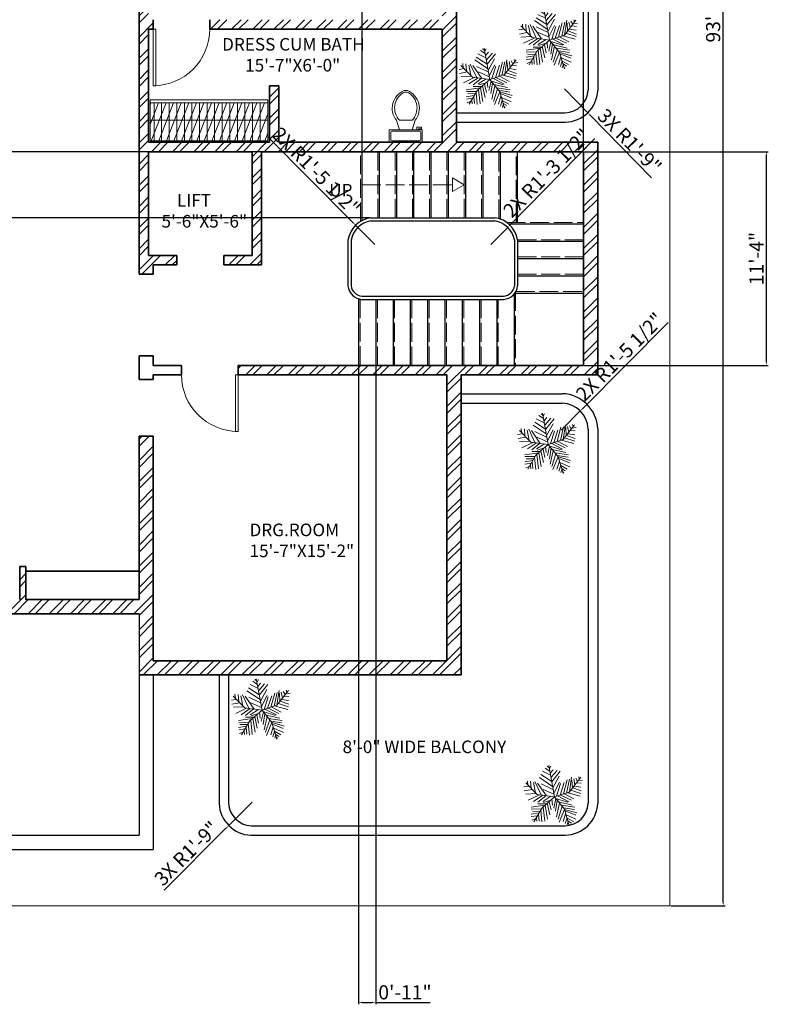
# Model space of a CAD drawing. Units: inches. Extents: x 155 to 1269, y 1260 to 2528.
# Tile 4 of 6: x 792 to 1269, y 1277 to 1903. Entities that reach past the tile are written whole.
import ezdxf

# ---------------------------------------------------------------- set-up
doc = ezdxf.new("R2010")
doc.units = ezdxf.units.IN
doc.linetypes.add('ACAD_ISO02W100', pattern=[15, 12, -3])
for name, color, linetype, lineweight in [('A-ANNO-DIMS', 2, 'Continuous', 18), ('A-ANNO-SYMB', 7, 'Continuous', 18), ('A-ANNO-TEXT', 7, 'Continuous', 25), ('A-AREA-IDEN', 7, 'Continuous', 18), ('A-DOOR', 3, 'Continuous', 18), ('A-FLOR-CASE', 9, 'Continuous', 18), ('A-FLOR-CASE-PATT', 252, 'Continuous', 13), ('A-FLOR-EDGE', 7, 'Continuous', 25), ('A-FLOR-FIXT', 9, 'Continuous', 18), ('A-FLOR-STRS', 7, 'Continuous', 25), ('A-FLOR-STRS-HIDN', 8, 'ACAD_ISO02W100', 13), ('A-FLOR-STRS-PATH', 7, 'ACAD_ISO02W100', 18), ('A-WALL', 7, 'Continuous', 35), ('A-WALL-PATT', 252, 'Continuous', 13), ('C-PROP', 8, 'Continuous', 18), ('L-PLNT', 94, 'Continuous', 13)]:
    doc.layers.add(name, color=color, linetype=linetype, lineweight=lineweight)
doc.styles.get("Standard").update_dxf_attribs({"font": 'arial.ttf'})
doc.dimstyles.new('ISO-25', dxfattribs={"dimtxt": 9, "dimasz": 2.5, "dimexe": 1.25, "dimexo": 0.625, "dimtad": 1, "dimlunit": 3, "dimtxsty": 'Standard', "dimcen": 2.5, "dimadec": 0, "dimazin": 0, "dimtfac": 1, "dimtmove": 0, "dimatfit": 3, "dimfxl": 1, "dimarcsym": 0})

# ---------------------------------------------------------------- blocks, each defined once
blk = doc.blocks.new('*U4')
for p, q in [((-40, 0), (-40, 6)), ((0, 0), (0, 6))]:
    blk.add_line(p, q)
blk.add_lwpolyline([(0, 0), (0, -40), (-1.75, -40), (-1.75, 0)], close=True)
blk.add_arc((0, 0), 40, 180, 270)
blk = doc.blocks.new('*U8')
for p, q in [((9.5, -6), (9.5, -2)), ((-10, -8.5), (-8, -8.5)), ((-10, -9.5), (-10, -8.5)), ((-7, -9.5), (-10, -9.5)), ((-8, -8.5), (-8, -8)), ((-7, -8), (-7, -9.5)), ((-4, -8), (-6, -14)), ((4, -8), (6, -14)), ((4, -14), (-4, -14))]:
    blk.add_line(p, q)
blk.add_lwpolyline([(10.5, -8), (10.5, 0), (-10.5, 0), (-10.5, -8)], close=True)
for points in [[(-9.5, -2), (-9.5, -6)], [(8.5, -1), (-8.5, -1)], [(-8.5, -7), (8.5, -7)]]:
    blk.add_lwpolyline(points)
for centre, radius, start, end in [((-8.62, -1.88), 0.884, 81.8699, 188.1301), ((-8.62, -6.12), 0.884, 171.8699, 278.1301), ((8.62, -1.88), 0.884, 351.8699, 98.1301), ((8.62, -6.12), 0.884, 261.8699, 8.1301), ((3.52, -21.58), 12.17, 141.46911, 247.97143), ((4.2, -21.82), 11.33, 136.36773, 238.94682), ((-3.52, -21.58), 12.17, 292.02843, 38.53071), ((-4.2, -21.82), 11.33, 301.05301, 43.63209), ((0, -27.88), 4, 245.73182, 294.26817), ((0, -29), 4, 254.86053, 285.13947)]:
    blk.add_arc(centre, radius, start, end)
blk = doc.blocks.new('*U9')
for p, q in [((0, 0), (0, 6)), ((40, 0), (40, 6))]:
    blk.add_line(p, q)
blk.add_lwpolyline([(0, 0), (0, -40), (1.75, -40), (1.75, 0)], close=True)
blk.add_arc((0, 0), 40, 270, 0)
blk = doc.blocks.new('*U11')
for p, q in [((-10.186, 53.64), (-13.084, 55.962)), ((0, 0), (-10.5, 57)), ((-9.099, 51.782), (-6.563, 55.962)), ((-5.114, 28.097), (-24.676, 40.636)), ((-7.288, 39.707), (-21.778, 46.673)), ((-8.737, 47.138), (-17.069, 52.711)), ((-7.65, 43.423), (-2.578, 49.46)), ((-5.839, 35.992), (4.667, 48.067)), ((-5.114, 27.632), (10.463, 46.673)), ((-2.941, 16.486), (8.652, 37.85)), ((27, 9), (48, 36)), ((27.127, 9.056), (31.112, 35.992)), ((44.153, 36.456), (45.239, 32.741)), ((-47.498, 19.737), (-55.83, 18.344)), ((-31.5, 4.5), (-52.5, 25.5)), ((-48.585, 21.131), (-49.309, 29.026)), ((-43.513, 28.561), (-42.427, 15.558)), ((-38.442, 26.239), (-34.819, 7.663)), ((-35.544, 28.097), (-24.314, 3.947)), ((-14.533, 2.09), (-30.834, 25.31)), ((-3.665, 19.273), (-27.574, 35.527)), ((-24.314, 23.917), (-2.941, 13.7)), ((-1.129, 6.734), (9.014, 26.704)), ((3.942, 1.625), (11.187, 24.381)), ((10.101, 3.483), (17.708, 26.239)), ((16.259, 5.805), (23.142, 31.348)), ((22.055, 7.198), (27.489, 32.277)), ((31.836, 30.883), (32.561, 16.486)), ((35.096, 32.741), (37.27, 22.524)), ((36.183, 19.737), (48.137, 17.88)), ((38.719, 34.134), (41.979, 28.561)), ((40.53, 25.775), (48.862, 24.846)), ((43.791, 29.954), (51.036, 30.883)), ((-40.615, 13.7), (-55.105, 10.913)), ((-33.37, 6.269), (-52.207, 5.34)), ((-28.299, 3.483), (-47.86, -5.805)), ((-21.416, 3.018), (-38.079, -8.128)), ((0, 0), (-31.5, 4.5)), ((-15.982, 2.09), (-30.11, -9.521)), ((0, 0), (-22.5, -19.5)), ((-6.563, 1.161), (-21.416, -8.128)), ((-20.691, 13.7), (-1.129, 4.876)), ((0, 0), (27, 9)), ((0, 0), (18, -22.5)), ((6.478, 1.625), (26.04, -8.592)), ((11.187, 3.483), (30.749, -5.805)), ((18.07, 5.805), (35.096, -3.483)), ((24.229, 7.663), (46.688, 1.625)), ((29.662, 12.307), (48.137, 6.269)), ((33.285, 16.486), (48.862, 10.913)), ((-17.431, -15.094), (-42.789, -18.809)), ((-15.257, -12.772), (-30.11, -12.772)), ((-6.563, -5.805), (-19.967, -9.985)), ((-17.069, -15.094), (-12.721, -40.172)), ((-13.446, -11.378), (-8.737, -32.741)), ((-9.461, -8.592), (-6.201, -23.453)), ((-4.752, -3.483), (-3.665, -14.629)), ((2.493, -3.019), (-1.491, -20.202)), ((1.769, -2.555), (24.229, -9.521)), ((5.029, -6.27), (2.131, -25.775)), ((9.014, -11.378), (3.58, -35.992)), ((14.085, -16.951), (6.478, -40.172)), ((7.565, -9.056), (32.198, -14.629)), ((12.274, -15.094), (36.907, -18.809)), ((-28.299, -29.026), (-42.789, -31.348)), ((-24.314, -21.596), (-42.427, -22.06)), ((-30.834, -34.135), (-42.427, -35.528)), ((-26.849, -26.24), (-40.253, -25.775)), ((-22.5, -19.5), (-37.5, -45)), ((-29.023, -30.884), (-27.936, -43.887)), ((-25.038, -23.918), (-22.865, -45.281)), ((-20.691, -18.345), (-17.793, -44.352)), ((18.07, -22.524), (8.289, -45.745)), ((20.244, -30.419), (15.897, -44.816)), ((16.259, -19.738), (36.183, -22.989)), ((18, -22.5), (27, -52.5)), ((18.433, -22.524), (40.53, -29.026)), ((19.157, -25.311), (38.719, -33.206)), ((21.331, -32.741), (39.081, -40.636)), ((-34.457, -39.708), (-40.978, -42.494)), ((-32.646, -36.921), (-31.921, -44.352)), ((22.78, -37.85), (19.519, -48.532)), ((22.78, -38.314), (34.372, -44.816)), ((24.591, -45.745), (23.142, -50.854)), ((24.591, -43.423), (30.749, -47.603)), ((26.764, -49.925), (28.213, -50.854))]:
    blk.add_line(p, q)
blk = doc.blocks.new('*D13')
at = {"layer": 'A-ANNO-DIMS', "color": 0, "lineweight": -2, "transparency": 16777216}
for p, q in [((1207.02, 2455.18), (1241.52, 2455.18)), ((1240.27, 1341.68), (1240.27, 2452.68)), ((1207.02, 1339.18), (1241.52, 1339.18))]:
    blk.add_line(p, q, dxfattribs=at)
at = {"layer": 'A-ANNO-DIMS', "color": 0, "transparency": 16777216}
for points in [[(1239.85, 2452.68), (1240.68, 2452.68), (1240.27, 2455.18)], [(1239.85, 1341.68), (1240.68, 1341.68), (1240.27, 1339.18)]]:
    blk.add_solid(points, dxfattribs=at)
at = {"layer": 'Defpoints', "color": 0, "transparency": 16777216}
for p in [(1206.4, 2455.18), (1240.27, 2455.18), (1206.4, 1339.18)]:
    blk.add_point(p, dxfattribs=at)
at = {"layer": 'A-ANNO-DIMS', "color": 0, "transparency": 16777216, "insert": (1235.04, 1897.18), "char_height": 9, "attachment_point": 5, "rotation": 90}
blk.add_mtext("93'", dxfattribs=at)
blk = doc.blocks.new('*D45')
at = {"layer": 'A-ANNO-DIMS', "color": 0, "lineweight": -2, "transparency": 16777216}
for p, q in [((1010.4, 1819.81), (1010.4, 2517.78)), ((1012.9, 2516.53), (1148.9, 2516.53)), ((1151.4, 1819.81), (1151.4, 2517.78))]:
    blk.add_line(p, q, dxfattribs=at)
at = {"layer": 'A-ANNO-DIMS', "color": 0, "transparency": 16777216}
for points in [[(1012.9, 2516.95), (1012.9, 2516.11), (1010.4, 2516.53)], [(1148.9, 2516.95), (1148.9, 2516.11), (1151.4, 2516.53)]]:
    blk.add_solid(points, dxfattribs=at)
at = {"layer": 'Defpoints', "color": 0, "transparency": 16777216}
for p in [(1151.4, 2516.53), (1010.4, 1819.18), (1151.4, 1819.18)]:
    blk.add_point(p, dxfattribs=at)
at = {"layer": 'A-ANNO-DIMS', "color": 0, "transparency": 16777216, "insert": (1080.9, 2521.75), "char_height": 9, "attachment_point": 5}
blk.add_mtext('11\'-9"', dxfattribs=at)
blk = doc.blocks.new('*D46')
at = {"layer": 'A-ANNO-DIMS', "color": 0, "lineweight": -2, "transparency": 16777216}
for p, q in [((1009.77, 1819.18), (164.8, 1819.18)), ((166.05, 1779.68), (166.05, 1816.68)), ((1015.06, 1777.18), (164.8, 1777.18))]:
    blk.add_line(p, q, dxfattribs=at)
at = {"layer": 'A-ANNO-DIMS', "color": 0, "transparency": 16777216}
for points in [[(165.63, 1816.68), (166.46, 1816.68), (166.05, 1819.18)], [(165.63, 1779.68), (166.46, 1779.68), (166.05, 1777.18)]]:
    blk.add_solid(points, dxfattribs=at)
at = {"layer": 'Defpoints', "color": 0, "transparency": 16777216}
for p in [(166.05, 1819.18), (1010.4, 1819.18), (1015.68, 1777.18)]:
    blk.add_point(p, dxfattribs=at)
at = {"layer": 'A-ANNO-DIMS', "color": 0, "transparency": 16777216, "insert": (160.82, 1798.18), "char_height": 9, "attachment_point": 5, "rotation": 90}
blk.add_mtext('3\'-6"', dxfattribs=at)
blk = doc.blocks.new('*D47')
at = {"layer": 'A-ANNO-DIMS', "color": 0, "lineweight": -2, "transparency": 16777216}
for p, q in [((1152.02, 1819.18), (1269, 1819.18)), ((1267.75, 1685.68), (1267.75, 1816.68)), ((1152.02, 1683.18), (1269, 1683.18))]:
    blk.add_line(p, q, dxfattribs=at)
at = {"layer": 'A-ANNO-DIMS', "color": 0, "transparency": 16777216}
for points in [[(1267.33, 1816.68), (1268.16, 1816.68), (1267.75, 1819.18)], [(1267.33, 1685.68), (1268.16, 1685.68), (1267.75, 1683.18)]]:
    blk.add_solid(points, dxfattribs=at)
at = {"layer": 'Defpoints', "color": 0, "transparency": 16777216}
for p in [(1151.4, 1819.18), (1267.75, 1819.18), (1151.4, 1683.18)]:
    blk.add_point(p, dxfattribs=at)
at = {"layer": 'A-ANNO-DIMS', "color": 0, "transparency": 16777216, "insert": (1262.6, 1751.18), "char_height": 9, "attachment_point": 5, "rotation": 90}
blk.add_mtext('11\'-4"', dxfattribs=at)
blk = doc.blocks.new('*D48')
at = {"layer": 'A-ANNO-DIMS', "color": 0, "lineweight": -2, "transparency": 16777216}
for p, q in [((1008.09, 1682.56), (1008.09, 1276.58)), ((1019.09, 1682.56), (1019.09, 1276.58)), ((1010.59, 1277.83), (1016.59, 1277.83)), ((1019.09, 1277.83), (1053.76, 1277.83))]:
    blk.add_line(p, q, dxfattribs=at)
at = {"layer": 'A-ANNO-DIMS', "color": 0, "transparency": 16777216}
for points in [[(1010.59, 1278.25), (1010.59, 1277.41), (1008.09, 1277.83)], [(1016.59, 1278.25), (1016.59, 1277.41), (1019.09, 1277.83)]]:
    blk.add_solid(points, dxfattribs=at)
at = {"layer": 'Defpoints', "color": 0, "transparency": 16777216}
for p in [(1008.09, 1683.18), (1019.09, 1683.18), (1019.09, 1277.83)]:
    blk.add_point(p, dxfattribs=at)
at = {"layer": 'A-ANNO-DIMS', "color": 0, "transparency": 16777216, "insert": (1037.68, 1283.05), "char_height": 9, "attachment_point": 5}
blk.add_mtext('0\'-11"', dxfattribs=at)
blk = doc.blocks.new('*D51')
at = {"layer": 'A-ANNO-DIMS', "color": 0, "lineweight": -2, "transparency": 16777216}
for p, q in [((1139.18, 1859.18), (1154.04, 1844.01)), ((1194.69, 1802.47), (1155.79, 1842.22))]:
    blk.add_line(p, q, dxfattribs=at)
at = {"layer": 'A-ANNO-DIMS', "color": 0, "transparency": 16777216}
blk.add_solid([(1156.08, 1842.51), (1155.49, 1841.93), (1154.04, 1844.01)], dxfattribs=at)
at = {"layer": 'Defpoints', "color": 0, "transparency": 16777216}
for p in [(1139.18, 1859.18), (1154.04, 1844.01)]:
    blk.add_point(p, dxfattribs=at)
at = {"layer": 'A-ANNO-DIMS', "color": 0, "transparency": 16777216, "insert": (1179.84, 1825.1), "char_height": 9, "attachment_point": 5, "rotation": 314.37911}
blk.add_mtext('3X R1\'-9"', dxfattribs=at)
blk = doc.blocks.new('*D52')
at = {"layer": 'A-ANNO-DIMS', "color": 0, "lineweight": -2, "transparency": 16777216}
for p, q in [((940.38, 1405.16), (925.51, 1390.34)), ((884.35, 1349.31), (923.74, 1388.57))]:
    blk.add_line(p, q, dxfattribs=at)
at = {"layer": 'A-ANNO-DIMS', "color": 0, "transparency": 16777216}
blk.add_solid([(923.45, 1388.87), (924.03, 1388.28), (925.51, 1390.34)], dxfattribs=at)
at = {"layer": 'Defpoints', "color": 0, "transparency": 16777216}
for p in [(940.38, 1405.16), (925.51, 1390.34)]:
    blk.add_point(p, dxfattribs=at)
at = {"layer": 'A-ANNO-DIMS', "color": 0, "transparency": 16777216, "insert": (899.47, 1371.76), "char_height": 9, "attachment_point": 5, "rotation": 44.90952}
blk.add_mtext('3X R1\'-9"', dxfattribs=at)
blk = doc.blocks.new('*D53')
at = {"layer": 'A-ANNO-DIMS', "color": 0, "lineweight": -2, "transparency": 16777216}
for p, q in [((950.39, 1828.55), (1004.51, 1774.13)), ((1018.54, 1760.02), (1006.27, 1772.36))]:
    blk.add_line(p, q, dxfattribs=at)
at = {"layer": 'A-ANNO-DIMS', "color": 0, "transparency": 16777216}
blk.add_solid([(1004.81, 1774.42), (1004.22, 1773.84), (1006.27, 1772.36)], dxfattribs=at)
at = {"layer": 'Defpoints', "color": 0, "transparency": 16777216}
for p in [(1006.27, 1772.36), (1018.54, 1760.02)]:
    blk.add_point(p, dxfattribs=at)
at = {"layer": 'A-ANNO-DIMS', "color": 0, "transparency": 16777216, "insert": (980.31, 1805.95), "char_height": 9, "attachment_point": 5, "rotation": 314.83905}
blk.add_mtext('2X R1\'-5 1/2"', dxfattribs=at)
blk = doc.blocks.new('*D54')
at = {"layer": 'A-ANNO-DIMS', "color": 0, "lineweight": -2, "transparency": 16777216}
for p, q in [((1205.15, 1710.39), (1151.06, 1655.94)), ((1137.09, 1641.87), (1149.3, 1654.16))]:
    blk.add_line(p, q, dxfattribs=at)
at = {"layer": 'A-ANNO-DIMS', "color": 0, "transparency": 16777216}
blk.add_solid([(1150.77, 1656.23), (1151.36, 1655.64), (1149.3, 1654.16)], dxfattribs=at)
at = {"layer": 'Defpoints', "color": 0, "transparency": 16777216}
for p in [(1149.3, 1654.16), (1137.09, 1641.87)]:
    blk.add_point(p, dxfattribs=at)
at = {"layer": 'A-ANNO-DIMS', "color": 0, "transparency": 16777216, "insert": (1175.24, 1687.77), "char_height": 9, "attachment_point": 5, "rotation": 45.19287}
blk.add_mtext('2X R1\'-5 1/2"', dxfattribs=at)
blk = doc.blocks.new('*D58')
at = {"layer": 'A-ANNO-DIMS', "color": 0, "lineweight": -2, "transparency": 16777216}
for p, q in [((1158.59, 1827.57), (1104.83, 1772.79)), ((1092.29, 1760.02), (1103.08, 1771.01))]:
    blk.add_line(p, q, dxfattribs=at)
at = {"layer": 'A-ANNO-DIMS', "color": 0, "transparency": 16777216}
blk.add_solid([(1104.53, 1773.08), (1105.12, 1772.5), (1103.08, 1771.01)], dxfattribs=at)
at = {"layer": 'Defpoints', "color": 0, "transparency": 16777216}
for p in [(1103.08, 1771.01), (1092.29, 1760.02)]:
    blk.add_point(p, dxfattribs=at)
at = {"layer": 'A-ANNO-DIMS', "color": 0, "transparency": 16777216, "insert": (1128.82, 1804.77), "char_height": 9, "attachment_point": 5, "rotation": 45.53236}
blk.add_mtext('2X R1\'-3 1/2"', dxfattribs=at)

msp = doc.modelspace()

# ---------------------------------------------------------------- hatches: boundary and pattern name
at = {"layer": 'A-FLOR-CASE-PATT'}
h = msp.add_hatch(dxfattribs=at)
h.set_pattern_fill('ANSI31', color=256, scale=1.4142, angle=23.5644, style=0)
h.paths.add_polyline_path([(875.397, 1826.181), (950.406, 1826.181), (950.406, 1850.181), (875.397, 1850.181)])
h = msp.add_hatch(dxfattribs=at)
h.set_pattern_fill('ANSI31', color=256, scale=1.51929, angle=45, style=0)
h.paths.add_polyline_path([(875.397, 1826.181), (950.406, 1826.181), (950.406, 1850.181), (875.397, 1850.181)])
at = {"layer": 'A-WALL-PATT'}
h = msp.add_hatch(dxfattribs=at)
h.set_pattern_fill('ANSI32', color=256)
h.paths.add_polyline_path([(614.897, 1534.181), (593.397, 1534.181), (593.397, 1555.181), (589.397, 1555.181), (589.397, 1534.181), (517.397, 1534.181), (517.397, 1555.181), (511.397, 1555.181), (511.397, 1495.181), (488.631, 1495.181), (488.631, 1486.181), (517.397, 1486.181), (517.397, 1525.181), (614.897, 1525.181)])
h.paths.add_polyline_path([(440.631, 1495.181), (344.954, 1495.181), (344.954, 1486.181), (440.631, 1486.181)])
h.paths.add_polyline_path([(323.954, 1495.181), (302.397, 1495.181), (302.397, 1625.863), (332.397, 1625.863), (332.397, 1631.863), (302.397, 1631.863), (302.397, 1634.984), (293.397, 1634.984), (293.397, 1486.181), (323.954, 1486.181)])
h.paths.add_polyline_path([(302.397, 1753.181), (386.397, 1753.181), (386.397, 1726.181), (392.397, 1726.181), (392.397, 1753.181), (511.397, 1753.181), (511.397, 1693.181), (392.397, 1693.181), (392.397, 1696.181), (386.397, 1696.181), (386.397, 1693.181), (368.397, 1693.181), (368.397, 1687.181), (511.397, 1687.181), (511.397, 1663.181), (517.397, 1663.181), (517.397, 1891.181), (539.397, 1891.181), (539.397, 1897.181), (517.397, 1897.181), (517.397, 2050.181), (511.397, 2050.181), (511.397, 1903.181), (374.397, 1903.181), (374.397, 1897.181), (410.397, 1897.181), (410.397, 1843.181), (416.397, 1843.181), (416.397, 1897.181), (511.397, 1897.181), (511.397, 1759.181), (416.397, 1759.181), (416.397, 1813.181), (410.397, 1813.181), (410.397, 1759.181), (302.397, 1759.181), (302.397, 1897.181), (338.397, 1897.181), (338.397, 1903.181), (302.397, 1903.181), (302.397, 1935.29), (293.397, 1935.29), (293.397, 1682.984), (302.397, 1682.984), (302.397, 1687.181), (338.397, 1687.181), (338.397, 1693.181), (302.397, 1693.181)])
h.paths.add_polyline_path([(645.397, 1897.181), (623.397, 1897.181), (623.397, 1891.181), (645.397, 1891.181)])
h.paths.add_polyline_path([(678.397, 1897.181), (669.397, 1897.181), (669.397, 1891.181), (678.397, 1891.181)])
h.paths.add_polyline_path([(696.397, 1897.181), (687.397, 1897.181), (687.397, 1891.181), (696.397, 1891.181)])
h.paths.add_polyline_path([(714.397, 1897.181), (705.397, 1897.181), (705.397, 1891.181), (714.397, 1891.181)])
h.paths.add_polyline_path([(732.397, 1897.181), (723.397, 1897.181), (723.397, 1891.181), (732.397, 1891.181)])
h.paths.add_polyline_path([(302.397, 2033.891), (293.397, 2033.891), (293.397, 1959.29), (302.397, 1959.29)], flags=17)
h.paths.add_polyline_path([(302.397, 2089.181), (511.397, 2089.181), (511.397, 2086.181), (517.397, 2086.181), (517.397, 2089.181), (527.397, 2089.181), (527.397, 2095.181), (302.397, 2095.181), (302.397, 2145.471), (293.397, 2145.471), (293.397, 2057.891), (302.397, 2057.891)])
h.paths.add_polyline_path([(773.397, 2095.181), (572.397, 2095.181), (572.397, 2308.181), (613.397, 2308.181), (613.397, 2443.181), (557.897, 2443.181), (557.897, 2434.181), (604.397, 2434.181), (604.397, 2314.181), (490.397, 2314.181), (490.397, 2359.181), (484.397, 2359.181), (484.397, 2314.181), (374.397, 2314.181), (374.397, 2308.181), (566.397, 2308.181), (566.397, 2095.181), (563.397, 2095.181), (563.397, 2089.181), (773.397, 2089.181)])
h.paths.add_polyline_path([(1070.397, 2147.681), (1061.397, 2147.681), (1061.397, 2095.181), (857.397, 2095.181), (857.397, 2089.181), (868.397, 2089.181), (868.397, 2086.181), (874.397, 2086.181), (874.397, 2089.181), (1061.397, 2089.181), (1061.397, 2050.181), (1070.397, 2050.181)])
h.paths.add_polyline_path([(821.397, 2095.181), (818.397, 2095.181), (818.397, 2308.181), (1022.397, 2308.181), (1022.397, 2314.181), (940.397, 2314.181), (940.397, 2434.181), (1077.397, 2434.181), (1077.397, 2389.181), (1083.397, 2389.181), (1083.397, 2434.181), (1129.897, 2434.181), (1129.897, 2443.181), (887.897, 2443.181), (887.897, 2434.181), (934.397, 2434.181), (934.397, 2314.181), (820.397, 2314.181), (820.397, 2359.181), (814.397, 2359.181), (814.397, 2314.181), (809.397, 2314.181), (809.397, 2308.181), (812.397, 2308.181), (812.397, 2095.181), (809.397, 2095.181), (809.397, 2089.181), (821.397, 2089.181)])
h.paths.add_polyline_path([(874.397, 2050.181), (868.397, 2050.181), (868.397, 1741.181), (877.397, 1741.181), (877.397, 1747.181), (892.397, 1747.181), (892.397, 1753.181), (874.397, 1753.181), (874.397, 1819.181), (940.397, 1819.181), (940.397, 1753.181), (922.397, 1753.181), (922.397, 1747.181), (946.397, 1747.181), (946.397, 1819.181), (1151.397, 1819.181), (1151.397, 1683.181), (931.397, 1683.181), (931.397, 1677.181), (1064.397, 1677.181), (1064.397, 1495.181), (877.397, 1495.181), (877.397, 1638.181), (868.397, 1638.181), (868.397, 1534.181), (796.397, 1534.181), (796.397, 1555.181), (792.397, 1555.181), (792.397, 1534.181), (770.897, 1534.181), (770.897, 1525.181), (868.397, 1525.181), (868.397, 1486.181), (1073.397, 1486.181), (1073.397, 1677.181), (1160.397, 1677.181), (1160.397, 1825.181), (1070.397, 1825.181), (1070.397, 1942.181), (1061.397, 1942.181), (1061.397, 1903.181), (913.397, 1903.181), (913.397, 1897.181), (1061.397, 1897.181), (1061.397, 1825.181), (957.406, 1825.181), (957.406, 1861.181), (951.406, 1861.181), (951.406, 1825.181), (874.397, 1825.181), (874.397, 1897.181), (877.397, 1897.181), (877.397, 1903.181), (874.397, 1903.181)])
h.paths.add_polyline_path([(1070.397, 2305.181), (1206.397, 2305.181), (1206.397, 2443.181), (1150.897, 2443.181), (1150.897, 2434.181), (1197.397, 2434.181), (1197.397, 2314.181), (1083.397, 2314.181), (1083.397, 2359.181), (1077.397, 2359.181), (1077.397, 2314.181), (1058.397, 2314.181), (1058.397, 2308.181), (1061.397, 2308.181), (1061.397, 2255.681), (1070.397, 2255.681)])
h.paths.add_polyline_path([(866.897, 2443.181), (673.397, 2443.181), (673.397, 2308.181), (773.397, 2308.181), (773.397, 2314.181), (682.397, 2314.181), (682.397, 2434.181), (814.397, 2434.181), (814.397, 2389.181), (818.897, 2389.181), (820.397, 2389.181), (820.397, 2434.181), (866.897, 2434.181)])
h.paths.add_polyline_path([(536.897, 2443.181), (293.397, 2443.181), (293.397, 2253.471), (302.397, 2253.471), (302.397, 2308.181), (338.397, 2308.181), (338.397, 2314.181), (302.397, 2314.181), (302.397, 2434.181), (484.397, 2434.181), (484.397, 2389.181), (490.397, 2389.181), (490.397, 2434.181), (536.897, 2434.181)])

# ---------------------------------------------------------------- linework, layer by layer
at = {"layer": 'A-ANNO-SYMB'}
msp.add_lwpolyline([(1075.397, 1798.181), (1067.963, 1802.473), (1067.963, 1793.889)], close=True, dxfattribs=at)
at = {"layer": 'A-FLOR-CASE'}
for p, q in [((875.397, 1852.181), (875.397, 1826.181)), ((875.397, 1852.181), (950.406, 1852.181)), ((875.397, 1850.181), (950.406, 1850.181)), ((950.406, 1852.181), (950.406, 1826.181)), ((875.397, 1839.181), (950.406, 1839.181)), ((875.397, 1826.181), (950.406, 1826.181))]:
    msp.add_line(p, q, dxfattribs=at)
at = {"layer": 'A-FLOR-EDGE'}
for p, q in [((1154.397, 2261.664), (1154.397, 1858.359)), ((1160.397, 2261.791), (1160.397, 1858.209)), ((1070.397, 1843.955), (1139.62, 1843.955)), ((1070.397, 1837.955), (1139.699, 1837.955)), ((1073.397, 1665.181), (1137.877, 1665.181)), ((1073.397, 1659.181), (1137.769, 1659.181)), ((1154.397, 1642.664), (1154.397, 1404.585)), ((1160.397, 1642.791), (1160.397, 1404.435)), ((868.397, 1525.181), (868.397, 1384.181)), ((877.397, 1486.181), (877.397, 1375.181)), ((919.397, 1486.181), (919.397, 1404.446)), ((925.397, 1486.181), (925.397, 1404.556)), ((939.719, 1390.181), (1139.62, 1390.181)), ((517.397, 1384.181), (868.397, 1384.181)), ((939.599, 1384.181), (1139.699, 1384.181)), ((508.397, 1375.181), (877.397, 1375.181))]:
    msp.add_line(p, q, dxfattribs=at)
for centre, radius, start, end in [((1139.185, 1859.184), 15.235, 271.638477, 356.895339), ((1139.185, 1859.184), 21.235, 271.387815, 357.37037), ((1137.094, 1641.873), 23.321, 2.254968, 88.076393), ((1137.094, 1641.873), 17.321, 2.616598, 87.767917), ((940.376, 1405.157), 20.991, 181.941445, 267.878551), ((940.376, 1405.157), 14.991, 182.2974, 267.489584), ((1139.185, 1405.41), 15.235, 271.638477, 356.895339), ((1139.185, 1405.41), 21.235, 271.387815, 357.37037)]:
    msp.add_arc(centre, radius, start, end, dxfattribs=at)
at = {"layer": 'A-FLOR-STRS'}
for p, q in [((1010.397, 1775.394), (1010.397, 1819.181)), ((1021.397, 1777.181), (1021.397, 1819.181)), ((1032.397, 1777.181), (1032.397, 1819.181)), ((1043.397, 1777.181), (1043.397, 1819.181)), ((1054.397, 1777.181), (1054.397, 1819.181)), ((1065.397, 1777.181), (1065.397, 1819.181)), ((1076.397, 1777.181), (1076.397, 1819.181)), ((1087.397, 1777.181), (1087.397, 1819.181)), ((1098.397, 1776.311), (1098.397, 1819.181)), ((1109.397, 1774.181), (1109.397, 1819.181)), ((1015.681, 1777.181), (1095.15, 1777.181)), ((1015.852, 1775.181), (1094.979, 1775.181)), ((1103.669, 1773.181), (1151.397, 1773.181)), ((1001.397, 1762.977), (1001.397, 1733.728)), ((1003.397, 1762.801), (1003.397, 1733.837)), ((1107.397, 1762.992), (1107.397, 1733.837)), ((1109.397, 1763.181), (1109.397, 1733.728)), ((1109.397, 1762.181), (1151.397, 1762.181)), ((1109.397, 1751.181), (1151.397, 1751.181)), ((1109.397, 1740.181), (1151.397, 1740.181)), ((1008.095, 1725.582), (1008.095, 1683.181)), ((1009.095, 1725.181), (1100.49, 1725.181)), ((1010.37, 1727.181), (1100.424, 1727.181)), ((1019.095, 1725.181), (1019.095, 1683.181)), ((1030.095, 1725.181), (1030.095, 1683.181)), ((1041.095, 1725.181), (1041.095, 1683.181)), ((1052.095, 1725.181), (1052.095, 1683.181)), ((1063.095, 1725.181), (1063.095, 1683.181)), ((1074.095, 1725.181), (1074.095, 1683.181)), ((1085.095, 1725.181), (1085.095, 1683.181)), ((1096.095, 1725.181), (1096.095, 1683.181)), ((1107.095, 1728.434), (1107.095, 1683.181)), ((1108.095, 1729.181), (1151.397, 1729.181))]:
    msp.add_line(p, q, dxfattribs=at)
for centre, radius, start, end in [((1018.539, 1760.022), 17.395, 99.456882, 170.219435), ((1018.539, 1760.022), 15.395, 100.053905, 169.60187), ((1092.292, 1760.022), 15.395, 11.122313, 79.946095), ((1092.292, 1760.022), 17.395, 10.461498, 80.543118), ((1010.895, 1734.711), 9.548, 185.907516, 266.459791), ((1010.895, 1734.711), 7.548, 186.645027, 266.018121), ((1099.9, 1734.711), 7.548, 273.981879, 353.354973), ((1099.9, 1734.711), 9.548, 273.540209, 354.092484)]:
    msp.add_arc(centre, radius, start, end, dxfattribs=at)
at = {"layer": 'A-FLOR-STRS-HIDN'}
for p, q in [((1009.397, 1774.821), (1009.397, 1819.181)), ((1020.397, 1777.181), (1020.397, 1819.181)), ((1031.397, 1777.181), (1031.397, 1819.181)), ((1042.397, 1777.181), (1042.397, 1819.181)), ((1053.397, 1777.181), (1053.397, 1819.181)), ((1064.397, 1777.181), (1064.397, 1819.181)), ((1075.397, 1777.181), (1075.397, 1819.181)), ((1086.397, 1777.181), (1086.397, 1819.181)), ((1097.397, 1776.651), (1097.397, 1819.181)), ((1108.397, 1774.181), (1108.397, 1819.181)), ((1102.397, 1774.181), (1151.397, 1774.181)), ((1109.397, 1763.181), (1151.397, 1763.181)), ((1109.397, 1752.181), (1151.397, 1752.181)), ((1109.397, 1741.181), (1151.397, 1741.181)), ((1108.095, 1729.811), (1108.095, 1683.181)), ((1108.305, 1730.181), (1151.397, 1730.181)), ((1009.095, 1725.334), (1009.095, 1683.181)), ((1020.095, 1725.181), (1020.095, 1683.181)), ((1031.095, 1725.181), (1031.095, 1683.181)), ((1042.095, 1725.181), (1042.095, 1683.181)), ((1053.095, 1725.181), (1053.095, 1683.181)), ((1064.095, 1725.181), (1064.095, 1683.181)), ((1075.095, 1725.181), (1075.095, 1683.181)), ((1086.095, 1725.181), (1086.095, 1683.181)), ((1097.095, 1725.181), (1097.095, 1683.181))]:
    msp.add_line(p, q, dxfattribs=at)
at = {"layer": 'A-FLOR-STRS-PATH'}
msp.add_line((1010.397, 1798.181), (1067.963, 1798.181), dxfattribs=at)
at = {"layer": 'A-WALL'}
for p, q in [((1070.397, 2305.181), (1070.397, 1825.181)), ((868.397, 2050.181), (868.397, 1741.181)), ((877.397, 1897.181), (877.397, 1903.181)), ((913.397, 1897.181), (913.397, 1903.181)), ((874.397, 1897.181), (874.397, 1825.181)), ((874.397, 1897.181), (877.397, 1897.181)), ((913.397, 1897.181), (1061.397, 1897.181)), ((1061.397, 1897.181), (1061.397, 1825.181)), ((957.406, 1861.181), (951.406, 1861.181)), ((951.406, 1861.181), (951.406, 1825.181)), ((957.406, 1825.181), (957.406, 1861.181)), ((874.397, 1825.181), (951.406, 1825.181)), ((957.406, 1825.181), (1061.397, 1825.181)), ((1070.397, 1825.181), (1160.397, 1825.181)), ((1160.397, 1825.181), (1160.397, 1677.181)), ((874.397, 1819.181), (874.397, 1753.181)), ((874.397, 1819.181), (940.397, 1819.181)), ((940.397, 1819.181), (940.397, 1753.181)), ((946.397, 1819.181), (946.397, 1747.181)), ((946.397, 1819.181), (1151.397, 1819.181)), ((1151.397, 1819.181), (1151.397, 1683.181)), ((874.397, 1753.181), (892.397, 1753.181)), ((892.397, 1753.181), (892.397, 1747.181)), ((922.397, 1753.181), (922.397, 1747.181)), ((922.397, 1753.181), (940.397, 1753.181)), ((877.397, 1747.181), (892.397, 1747.181)), ((877.397, 1747.181), (877.397, 1741.181)), ((922.397, 1747.181), (946.397, 1747.181)), ((877.397, 1741.181), (868.397, 1741.181)), ((877.397, 1689.181), (868.397, 1689.181)), ((868.397, 1689.181), (868.397, 1674.181)), ((877.397, 1689.181), (877.397, 1683.181)), ((877.397, 1683.181), (895.397, 1683.181)), ((895.397, 1677.181), (895.397, 1683.181)), ((931.397, 1677.181), (931.397, 1683.181)), ((931.397, 1683.181), (1151.397, 1683.181)), ((877.397, 1674.181), (868.397, 1674.181)), ((877.397, 1677.181), (895.397, 1677.181)), ((877.397, 1677.181), (877.397, 1674.181)), ((931.397, 1677.181), (1064.397, 1677.181)), ((1064.397, 1677.181), (1064.397, 1495.181)), ((1073.397, 1677.181), (1073.397, 1486.181)), ((1073.397, 1677.181), (1160.397, 1677.181)), ((877.397, 1638.181), (868.397, 1638.181)), ((868.397, 1638.181), (868.397, 1534.181)), ((877.397, 1638.181), (877.397, 1495.181)), ((796.397, 1555.181), (792.397, 1555.181)), ((792.397, 1555.181), (792.397, 1534.181)), ((796.397, 1555.181), (796.397, 1534.181)), ((796.397, 1552.181), (868.397, 1552.181)), ((796.397, 1534.181), (868.397, 1534.181)), ((517.397, 1525.181), (868.397, 1525.181)), ((877.397, 1495.181), (1064.397, 1495.181)), ((868.397, 1486.181), (1073.397, 1486.181))]:
    msp.add_line(p, q, dxfattribs=at)
at = {"layer": 'C-PROP'}
for p in [(1206.397, 2305.181), (227.397, 1339.181)]:
    msp.add_line(p, (1206.397, 1339.181), dxfattribs=at)

# ---------------------------------------------------------------- block references
at = {"layer": 'A-DOOR', "xscale": 0.9, "yscale": 0.9, "zscale": 0.9}
for name, p in [('*U9', (877.397, 1897.181)), ('*U4', (931.397, 1677.181))]:
    msp.add_blockref(name, p, dxfattribs=at)
at = {"layer": 'A-FLOR-FIXT', "rotation": 180}
msp.add_blockref('*U8', (1038.217, 1825.181), dxfattribs=at)
at = {"layer": 'L-PLNT', "xscale": 0.3495173552522817, "yscale": 0.3495173552522817, "zscale": 0.3495173552522817}
for p in [(1129.772, 1890.256), (1091.697, 1865.126), (1128.907, 1632.818), (946.697, 1463.73), (1132.874, 1408.531)]:
    msp.add_blockref('*U11', p, dxfattribs=at)

# ---------------------------------------------------------------- texts
at = {"layer": 'A-ANNO-TEXT', "insert": (989.447, 1798.683), "char_height": 8, "attachment_point": 1}
msp.add_mtext_dynamic_manual_height_columns('UP', width=15.15571, gutter_width=12.5, heights=[0], dxfattribs=at)
at = {"layer": 'A-AREA-IDEN', "char_height": 8, "attachment_point": 1}
for s, width, insert in [('DRESS CUM BATH\\P      15\'-7"X6\'-0"', 98.45802, (921.275, 1891.514)), ('    LIFT 5\'-6"X5\'-6"', 53.61629, (882.7, 1792.221)), ('DRG.ROOM 15\'-7"X15\'-2"', 64.53356, (938.731, 1582.493)), ('8\'-0" WIDE BALCONY', 110.88305, (997.979, 1444.437))]:
    msp.add_mtext_dynamic_manual_height_columns(s, width=width, gutter_width=12.5, heights=[0], dxfattribs=dict(at, insert=insert))

# ---------------------------------------------------------------- dimensions: what is measured, and where the dimension line sits
at = {"layer": 'A-ANNO-DIMS'}
for base, p1, p2, picture, middle in [((1151.397, 2516.531), (1010.397, 1819.181), (1151.397, 1819.181), '*D45', (1080.897, 2521.751)), ((1019.095, 1277.831), (1008.095, 1683.181), (1019.095, 1683.181), '*D48', (1037.678, 1283.051))]:
    dim = msp.add_linear_dim(base=base, p1=p1, p2=p2, dimstyle='ISO-25', override={"dimdec": 1, "dimlfac": 1, "dimrnd": 0, "dimzin": 1, "dimdsep": 46, "dimlunit": 4, "dimfrac": 2}, dxfattribs=at)
    dim.commit()
    dim.dimension.update_dxf_attribs({"geometry": picture, "text_midpoint": middle})
for base, p1, p2, override, picture, middle in [((1240.268, 2455.181), (1206.397, 1339.181), (1206.397, 2455.181), {"dimclrd": 0, "dimclre": 0, "dimclrt": 0}, '*D13', (1235.044, 1897.181)), ((166.047, 1819.181), (1015.681, 1777.181), (1010.397, 1819.181), {"dimdec": 1, "dimlfac": 1, "dimrnd": 0, "dimzin": 1, "dimdsep": 46, "dimlunit": 4, "dimfrac": 2}, '*D46', (160.824, 1798.181)), ((1267.747, 1819.181), (1151.397, 1683.181), (1151.397, 1819.181), {"dimdec": 1, "dimlfac": 1, "dimrnd": 0, "dimzin": 1, "dimdsep": 46, "dimlunit": 4, "dimfrac": 2}, '*D47', (1262.604, 1751.181))]:
    dim = msp.add_linear_dim(base=base, p1=p1, p2=p2, angle=90, dimstyle='ISO-25', override=override, dxfattribs=at)
    dim.commit()
    dim.dimension.update_dxf_attribs({"geometry": picture, "text_midpoint": middle})
for center, mpoint, text, picture, middle in [((1139.185, 1859.184), (1154.037, 1844.006), '3X <>', '*D51', (1179.843, 1825.103)), ((1018.539, 1760.022), (1006.274, 1772.357), '2X <>', '*D53', (980.314, 1805.95)), ((1092.292, 1760.022), (1103.076, 1771.009), '2X <>', '*D58', (1128.816, 1804.771)), ((1137.094, 1641.873), (1149.301, 1654.162), '2X <>', '*D54', (1175.243, 1687.769)), ((940.376, 1405.157), (925.51, 1390.338), '3X <>', '*D52', (899.471, 1371.756))]:
    dim = msp.add_radius_dim(center=center, mpoint=mpoint, text=text, dimstyle='ISO-25', override={"dimdec": 1, "dimlfac": 1, "dimrnd": 0, "dimzin": 1, "dimdsep": 46, "dimlunit": 4, "dimfrac": 2}, dxfattribs=at)
    dim.commit()
    dim.dimension.update_dxf_attribs({"geometry": picture, "text_midpoint": middle})

doc.saveas('drawing.dxf')
